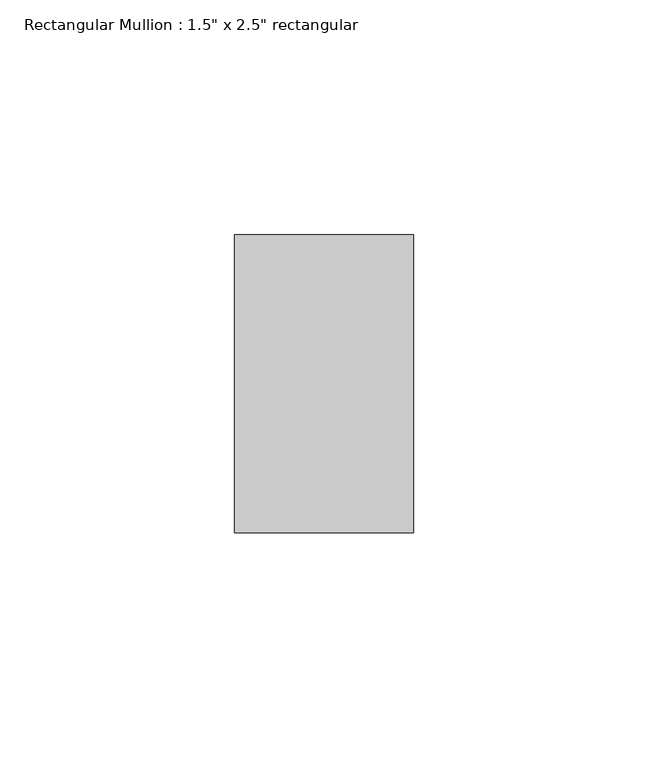
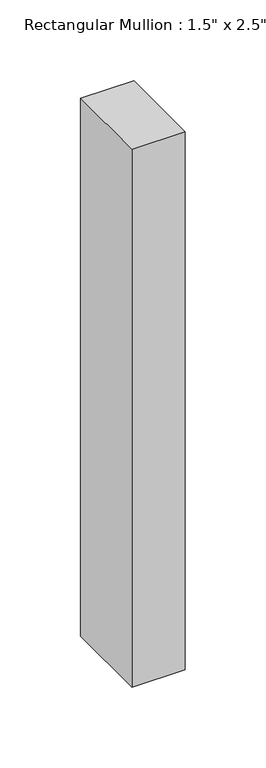
"""IFC4 building model written with IfcOpenShell, lengths in millimetres: member geometry."""

from ifc_helpers import new_model, si_unit, frame, origin, place, context, project, spatial, polyline, outline, extrude, source, transform, mapped, element, save


def member_711dd202(model_context):
    return source(origin(), model_context, "Body", "SweptSolid", [
        extrude(outline(polyline([(0.0, 31.75), (0.0, -31.75), (-38.1, -31.75), (-38.1, 31.75), (0.0, 31.75)])), frame((0.0, 0.0, -406.4), z_axis=(0.0, 0.0, 1.0), x_axis=(1.0, 0.0, 0.0)), (0.0, 0.0, 1.0), 406.4),
    ])


if __name__ == "__main__":
    model = new_model("IFC4")
    model_context = context("Model", 3, world=origin())
    ifc_project = project(units=[si_unit("LENGTHUNIT", "METRE", prefix="MILLI")], contexts=[model_context])
    site = spatial("IfcSite", under=ifc_project)
    building = spatial("IfcBuilding", under=site)
    placement = place(None, origin())
    member_shape = member_711dd202(model_context)
    element("IfcMember", 1, ObjectType="Rectangular Mullion : 1.5\" x 2.5\" rectangular", at=placement, inside=building, context=model_context, shape_type="MappedRepresentation", body=[
        mapped(member_shape, transform((0.0, 0.0, 0.0), x_axis=(1.0, 0.0, 0.0), y_axis=(0.0, 1.0, 0.0), z_axis=(0.0, 0.0, 1.0))),
    ])
    save(model, "model.ifc")

# Revit data of these elements
# Type "Rectangular Mullion : 1.5\" x 2.5\" rectangular"
#   built-in parameter 1007304 = 0.208333 (stored number, unit not read)
#   built-in parameter 1007301 = 0.0625 (stored number, unit not read)
#   built-in parameter 1007300 = 0.0625 (stored number, unit not read)
# Element 1 (IfcMember, "Rectangular Mullion : 1.5\" x 2.5\" rectangular")
#   Materials on its faces: "Damp-proofing"
# Materials
#   "Damp-proofing": class "Generic", colour RGB 127 127 127, transparency 0, Description = "Damp-proofing", Cost = 0
